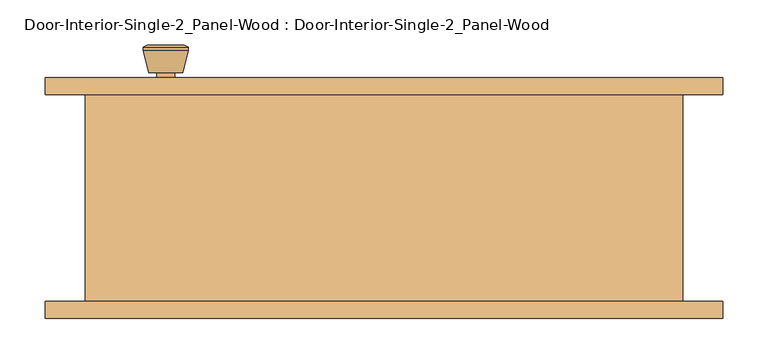
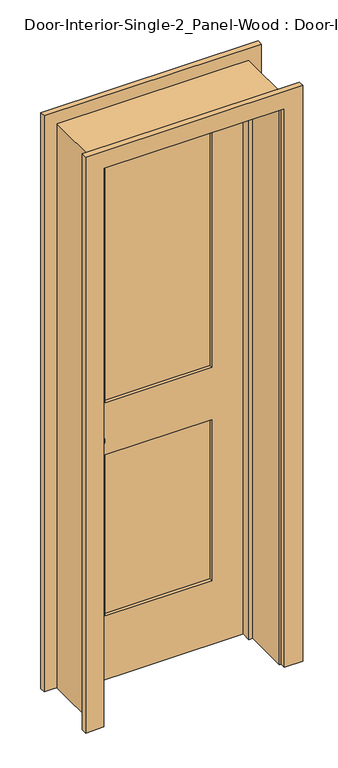
"""IFC4 building model written with IfcOpenShell, lengths in millimetres: door geometry, Door-Interior-Single-2_Panel-Wood : Door-Interior-Single-2_Panel-Wood."""

from ifc_helpers import new_model, si_unit, point, frame, frame_2d, origin, place, context, project, spatial, polyline, circle_curve, trimmed, segment, composite_curve, outline, extrude, faceted_brep, source, transform, mapped, element, save
from ifc_brep_helpers import plane_surface, cylinder_surface, revolved_surface, advanced_brep


def door_interior_single_2_panel_wood_door_interior_single_2_5f4e2ecc(model_context):
    return source(origin(), model_context, "Body", "SolidModel", [
        advanced_brep(
        [(-241.3, 70.2, 914.4), (-231.3, 70.2, 914.4), (-251.3, 70.2, 914.4), (-220.8241324, 21.2, 914.4), (-241.3, 21.2, 914.4), (-261.7758676, 21.2, 914.4), (-216.3, 23.0278681, 914.4), (-266.3, 23.0278681, 914.4), (-216.3, 26.4915463, 914.4), (-266.3, 26.4915463, 914.4), (-222.663764, 51.2, 914.4), (-259.936236, 51.2, 914.4), (-231.3, 51.2, 914.4), (-251.3, 51.2, 914.4)],
        [
            (0, 1),
            (1, 2, circle_curve(frame((-241.3, 70.2, 914.4), z_axis=(0.0, 1.0, 0.0), x_axis=(-1.0, 0.0, 0.0)), 10.0)),
            (2, 0),
            (2, 1, circle_curve(frame((-241.3, 70.2, 914.4), z_axis=(0.0, 1.0, 0.0), x_axis=(-1.0, 0.0, 0.0)), 10.0)),
            (3, 4),
            (4, 5),
            (5, 3, circle_curve(frame((-241.3, 21.2, 914.4), z_axis=(0.0, -1.0, 0.0), x_axis=(-1.0, 0.0, 0.0)), 20.4758676)),
            (3, 5, circle_curve(frame((-241.3, 21.2, 914.4), z_axis=(0.0, -1.0, 0.0), x_axis=(-1.0, 0.0, 0.0)), 20.4758676)),
            (6, 3),
            (5, 7),
            (7, 6, circle_curve(frame((-241.3, 23.0278681, 914.4), z_axis=(0.0, -1.0, 0.0), x_axis=(-1.0, 0.0, 0.0)), 25.0)),
            (6, 7, circle_curve(frame((-241.3, 23.0278681, 914.4), z_axis=(0.0, -1.0, 0.0), x_axis=(-1.0, 0.0, 0.0)), 25.0)),
            (8, 6),
            (7, 9),
            (9, 8, circle_curve(frame((-241.3, 26.4915463, 914.4), z_axis=(0.0, -1.0, 0.0), x_axis=(-1.0, 0.0, 0.0)), 25.0)),
            (8, 9, circle_curve(frame((-241.3, 26.4915463, 914.4), z_axis=(0.0, -1.0, 0.0), x_axis=(-1.0, 0.0, 0.0)), 25.0)),
            (10, 8),
            (9, 11),
            (11, 10, circle_curve(frame((-241.3, 51.2, 914.4), z_axis=(0.0, -1.0, 0.0), x_axis=(-1.0, 0.0, 0.0)), 18.636236)),
            (10, 11, circle_curve(frame((-241.3, 51.2, 914.4), z_axis=(0.0, -1.0, 0.0), x_axis=(-1.0, 0.0, 0.0)), 18.636236)),
            (12, 10),
            (11, 13),
            (13, 12, circle_curve(frame((-241.3, 51.2, 914.4), z_axis=(0.0, -1.0, 0.0), x_axis=(-1.0, 0.0, 0.0)), 10.0)),
            (12, 13, circle_curve(frame((-241.3, 51.2, 914.4), z_axis=(0.0, -1.0, 0.0), x_axis=(-1.0, 0.0, 0.0)), 10.0)),
            (1, 12),
            (13, 2),
        ],
        [
            plane_surface(frame((-241.3, 70.2, 914.4), z_axis=(0.0, 1.0, 0.0), x_axis=(-1.0, 0.0, 0.0))),
            plane_surface(frame((-241.3, 21.2, 914.4), z_axis=(0.0, -1.0, 0.0), x_axis=(-1.0, 0.0, 0.0))),
            revolved_surface(polyline([(-261.7758676, 21.2, 914.4), (-266.3, 23.0278681, 914.4)]), (-241.3, 70.2, 914.4), (0.0, 1.0, 0.0)),
            cylinder_surface(frame((-241.3, 70.2, 914.4), z_axis=(0.0, 1.0, 0.0), x_axis=(-1.0, 0.0, 0.0)), 25.0),
            revolved_surface(polyline([(-266.3, 26.4915463, 914.4), (-259.936236, 51.2, 914.4)]), (-241.3, 70.2, 914.4), (0.0, 1.0, 0.0)),
            plane_surface(frame((-241.3, 51.2, 914.4), z_axis=(0.0, 1.0, 0.0), x_axis=(-1.0, 0.0, 0.0))),
            cylinder_surface(frame((-241.3, 70.2, 914.4), z_axis=(0.0, 1.0, 0.0), x_axis=(-1.0, 0.0, 0.0)), 10.0),
        ],
        [
            (0, [[1, 2, 3]]),
            (0, [[-3, 4, -1]]),
            (1, [[5, 6, 7]]),
            (1, [[-6, -5, 8]]),
            (2, [[9, -7, 10, 11]]),
            (2, [[-10, -8, -9, 12]]),
            (3, [[13, -11, 14, 15]]),
            (3, [[-14, -12, -13, 16]]),
            (4, [[17, -15, 18, 19]]),
            (4, [[-18, -16, -17, 20]]),
            (5, [[21, -19, 22, 23]]),
            (5, [[-22, -20, -21, 24]]),
            (6, [[25, -23, 26, -2]]),
            (6, [[-26, -24, -25, -4]]),
        ],
    ),
        extrude(outline(composite_curve([segment(trimmed(circle_curve(frame_2d((914.4, -241.3)), 30.0), [point((914.4, -271.3))], [point((914.4, -211.3))], False, "CARTESIAN"), True, "CONTINUOUS"), segment(trimmed(circle_curve(frame_2d((914.4, -241.3)), 30.0), [point((914.4, -211.3))], [point((914.4, -271.3))], False, "CARTESIAN"), True, "CONTINUOUS")], self_intersect=False)), frame((0.0, 70.2, 0.0), z_axis=(0.0, 1.0, 0.0), x_axis=(0.0, 0.0, 1.0)), (0.0, 0.0, 1.0), 6.0),
        advanced_brep(
        [(-241.3, 117.125, 914.4), (-251.3, 117.125, 914.4), (-231.3, 117.125, 914.4), (-220.8241324, 166.125, 914.4), (-261.7758676, 166.125, 914.4), (-241.3, 166.125, 914.4), (-216.3, 164.2971319, 914.4), (-266.3, 164.2971319, 914.4), (-216.3, 160.8334537, 914.4), (-266.3, 160.8334537, 914.4), (-222.663764, 136.125, 914.4), (-259.936236, 136.125, 914.4), (-231.3, 136.125, 914.4), (-251.3, 136.125, 914.4)],
        [
            (0, 1),
            (1, 2, circle_curve(frame((-241.3, 117.125, 914.4), z_axis=(0.0, -1.0, 0.0), x_axis=(-1.0, 0.0, 0.0)), 10.0)),
            (2, 0),
            (2, 1, circle_curve(frame((-241.3, 117.125, 914.4), z_axis=(0.0, -1.0, 0.0), x_axis=(-1.0, 0.0, 0.0)), 10.0)),
            (3, 4, circle_curve(frame((-241.3, 166.125, 914.4), z_axis=(0.0, 1.0, 0.0), x_axis=(-1.0, 0.0, 0.0)), 20.4758676)),
            (4, 5),
            (5, 3),
            (4, 3, circle_curve(frame((-241.3, 166.125, 914.4), z_axis=(0.0, 1.0, 0.0), x_axis=(-1.0, 0.0, 0.0)), 20.4758676)),
            (6, 7, circle_curve(frame((-241.3, 164.2971319, 914.4), z_axis=(0.0, 1.0, 0.0), x_axis=(-1.0, 0.0, 0.0)), 25.0)),
            (7, 4),
            (3, 6),
            (7, 6, circle_curve(frame((-241.3, 164.2971319, 914.4), z_axis=(0.0, 1.0, 0.0), x_axis=(-1.0, 0.0, 0.0)), 25.0)),
            (8, 9, circle_curve(frame((-241.3, 160.8334537, 914.4), z_axis=(0.0, 1.0, 0.0), x_axis=(-1.0, 0.0, 0.0)), 25.0)),
            (9, 7),
            (6, 8),
            (9, 8, circle_curve(frame((-241.3, 160.8334537, 914.4), z_axis=(0.0, 1.0, 0.0), x_axis=(-1.0, 0.0, 0.0)), 25.0)),
            (10, 11, circle_curve(frame((-241.3, 136.125, 914.4), z_axis=(0.0, 1.0, 0.0), x_axis=(-1.0, 0.0, 0.0)), 18.636236)),
            (11, 9),
            (8, 10),
            (11, 10, circle_curve(frame((-241.3, 136.125, 914.4), z_axis=(0.0, 1.0, 0.0), x_axis=(-1.0, 0.0, 0.0)), 18.636236)),
            (12, 13, circle_curve(frame((-241.3, 136.125, 914.4), z_axis=(0.0, 1.0, 0.0), x_axis=(-1.0, 0.0, 0.0)), 10.0)),
            (13, 11),
            (10, 12),
            (13, 12, circle_curve(frame((-241.3, 136.125, 914.4), z_axis=(0.0, 1.0, 0.0), x_axis=(-1.0, 0.0, 0.0)), 10.0)),
            (1, 13),
            (12, 2),
        ],
        [
            plane_surface(frame((-241.3, 117.125, 914.4), z_axis=(0.0, -1.0, 0.0), x_axis=(-1.0, 0.0, 0.0))),
            plane_surface(frame((-241.3, 166.125, 914.4), z_axis=(0.0, 1.0, 0.0), x_axis=(-1.0, 0.0, 0.0))),
            revolved_surface(polyline([(-261.7758676, 166.125, 914.4), (-266.3, 164.2971319, 914.4)]), (-241.3, 117.125, 914.4), (0.0, -1.0, 0.0)),
            cylinder_surface(frame((-241.3, 117.125, 914.4), z_axis=(0.0, -1.0, 0.0), x_axis=(-1.0, 0.0, 0.0)), 25.0),
            revolved_surface(polyline([(-266.3, 160.8334537, 914.4), (-259.936236, 136.125, 914.4)]), (-241.3, 117.125, 914.4), (0.0, -1.0, 0.0)),
            plane_surface(frame((-241.3, 136.125, 914.4), z_axis=(0.0, -1.0, 0.0), x_axis=(-1.0, 0.0, 0.0))),
            cylinder_surface(frame((-241.3, 117.125, 914.4), z_axis=(0.0, -1.0, 0.0), x_axis=(-1.0, 0.0, 0.0)), 10.0),
        ],
        [
            (0, [[1, 2, 3]]),
            (0, [[-3, 4, -1]]),
            (1, [[5, 6, 7]]),
            (1, [[8, -7, -6]]),
            (2, [[9, 10, -5, 11]]),
            (2, [[12, -11, -8, -10]]),
            (3, [[13, 14, -9, 15]]),
            (3, [[16, -15, -12, -14]]),
            (4, [[17, 18, -13, 19]]),
            (4, [[20, -19, -16, -18]]),
            (5, [[21, 22, -17, 23]]),
            (5, [[24, -23, -20, -22]]),
            (6, [[-2, 25, -21, 26]]),
            (6, [[-4, -26, -24, -25]]),
        ],
    ),
        extrude(outline(composite_curve([segment(trimmed(circle_curve(frame_2d((914.4, -241.3)), 30.0), [point((914.4, -271.3))], [point((914.4, -211.3))], False, "CARTESIAN"), True, "CONTINUOUS"), segment(trimmed(circle_curve(frame_2d((914.4, -241.3)), 30.0), [point((914.4, -211.3))], [point((914.4, -271.3))], False, "CARTESIAN"), True, "CONTINUOUS")], self_intersect=False)), frame((0.0, 111.125, 0.0), z_axis=(0.0, 1.0, 0.0), x_axis=(0.0, 0.0, 1.0)), (0.0, 0.0, 1.0), 6.0),
        faceted_brep([(330.2, 111.125, 0.0), (330.2, -117.475, 0.0), (304.8, -117.475, 0.0), (304.8, 41.275, 0.0), (292.1, 41.275, 0.0), (292.1, 76.2, 0.0), (304.8, 76.2, 0.0), (304.8, 111.125, 0.0), (330.2, 111.125, 2057.4), (330.2, -117.475, 2057.4), (-330.2, -117.475, 2057.4), (-330.2, -117.475, 0.0), (-304.8, -117.475, 0.0), (-304.8, -117.475, 2032.0), (304.8, -117.475, 2032.0), (304.8, 41.275, 2032.0), (-304.8, 41.275, 2032.0), (-304.8, 41.275, 0.0), (-292.1, 41.275, 0.0), (-292.1, 41.275, 2019.3), (292.1, 41.275, 2019.3), (292.1, 76.2, 2019.3), (-292.1, 76.2, 2019.3), (-292.1, 76.2, 0.0), (-304.8, 76.2, 0.0), (-304.8, 76.2, 2032.0), (304.8, 76.2, 2032.0), (304.8, 111.125, 2032.0), (-304.8, 111.125, 2032.0), (-304.8, 111.125, 0.0), (-330.2, 111.125, 0.0), (-330.2, 111.125, 2057.4)], [[[0, 1, 2, 3, 4, 5, 6, 7]], [[1, 0, 8, 9]], [[2, 1, 9, 10, 11, 12, 13, 14]], [[3, 2, 14, 15]], [[4, 3, 15, 16, 17, 18, 19, 20]], [[5, 4, 20, 21]], [[6, 5, 21, 22, 23, 24, 25, 26]], [[7, 6, 26, 27]], [[0, 7, 27, 28, 29, 30, 31, 8]], [[9, 8, 31, 10]], [[15, 14, 13, 16]], [[21, 20, 19, 22]], [[27, 26, 25, 28]], [[30, 29, 24, 23, 18, 17, 12, 11]], [[10, 31, 30, 11]], [[16, 13, 12, 17]], [[22, 19, 18, 23]], [[28, 25, 24, 29]]]),
        extrude(outline(polyline([(2032.0, -304.8), (0.0, -304.8), (0.0, 304.8), (2032.0, 304.8), (2032.0, -304.8)]), holes=[polyline([(1912.9375, -184.15), (1912.9375, 184.15), (1009.65, 184.15), (1009.65, -184.15), (1912.9375, -184.15)]), polyline([(819.15, -184.15), (819.15, 184.15), (231.775, 184.15), (231.775, -184.15), (819.15, -184.15)])]), frame((0.0, 76.2, 0.0), z_axis=(0.0, 1.0, 0.0), x_axis=(0.0, 0.0, 1.0)), (0.0, 0.0, 1.0), 34.925),
        extrude(outline(polyline([(184.15, 87.8416667), (-184.15, 87.8416667), (-184.15, 99.4833333), (184.15, 99.4833333), (184.15, 87.8416667)])), frame((0.0, 0.0, 1009.65), z_axis=(0.0, 0.0, 1.0), x_axis=(1.0, 0.0, 0.0)), (0.0, 0.0, 1.0), 903.2875),
        extrude(outline(polyline([(184.15, 87.8416667), (-184.15, 87.8416667), (-184.15, 99.4833333), (184.15, 99.4833333), (184.15, 87.8416667)])), frame((0.0, 0.0, 231.775), z_axis=(0.0, 0.0, 1.0), x_axis=(1.0, 0.0, 0.0)), (0.0, 0.0, 1.0), 587.375),
        extrude(outline(polyline([(0.0, 311.15), (0.0, 374.65), (2101.85, 374.65), (2101.85, -374.65), (0.0, -374.65), (0.0, -311.15), (2038.35, -311.15), (2038.35, 311.15), (0.0, 311.15)])), frame((0.0, 111.125, 0.0), z_axis=(0.0, 1.0, 0.0), x_axis=(0.0, 0.0, 1.0)), (0.0, 0.0, 1.0), 19.05),
        extrude(outline(polyline([(0.0, 311.15), (0.0, 374.65), (2101.85, 374.65), (2101.85, -374.65), (0.0, -374.65), (0.0, -311.15), (2038.35, -311.15), (2038.35, 311.15), (0.0, 311.15)])), frame((0.0, -136.525, 0.0), z_axis=(0.0, 1.0, 0.0), x_axis=(0.0, 0.0, 1.0)), (0.0, 0.0, 1.0), 19.05),
    ])


if __name__ == "__main__":
    model = new_model("IFC4")
    model_context = context("Model", 3, world=origin())
    ifc_project = project(units=[si_unit("LENGTHUNIT", "METRE", prefix="MILLI")], contexts=[model_context])
    site = spatial("IfcSite", under=ifc_project)
    building = spatial("IfcBuilding", under=site)
    placement = place(None, origin())
    door_interior_single_2_panel_wood_door_interior_single_2_shape = door_interior_single_2_panel_wood_door_interior_single_2_5f4e2ecc(model_context)
    element("IfcDoor", 1, ObjectType="Door-Interior-Single-2_Panel-Wood : Door-Interior-Single-2_Panel-Wood", at=placement, inside=building, context=model_context, shape_type="MappedRepresentation", body=[
        mapped(door_interior_single_2_panel_wood_door_interior_single_2_shape, transform((0.0, 0.0, 0.0), x_axis=(1.0, 0.0, 0.0), y_axis=(0.0, 1.0, 0.0), z_axis=(0.0, 0.0, 1.0))),
    ])
    save(model, "model.ifc")

# Revit data of these elements
# Type "Door-Interior-Single-2_Panel-Wood : Door-Interior-Single-2_Panel-Wood"
#   Type Mark = "12"
#   Assembly Code = "C1020300"
#   Analytic Construction = "Wooden"
#   Top Rail = 0' - 4 11/16"
#   Thickness = 0' - 1 3/8"
#   Thermal Resistance (R) = 2.5876 (h·ft²·°F)/BTU
#   Swing Angle [instance default] = 90.00°
#   Stiles = 0' - 4 3/4"
#   Rough Width = 2' - 2"
#   Rough Height = 6' - 9"
#   Lock Rail = 0' - 7 1/2"
#   Height = 6' - 8"
#   Width = 2' - 0"
#   Heat Transfer Coefficient (U) = 0.3865 BTU/(h·ft²·°F)
#   Bottom Rail = 0' - 9 1/8"
#   Trim Material = Cherry
#   Panel Material = Cherry
#   Frame Material = Cherry
#   Door Handle Material = Aluminum
#   Visual Light Transmittance = 0
#   Solar Heat Gain Coefficient = 0
#   Wall Closure = (empty or 0)
#   Function = (empty or 0)
# Element 1 (IfcDoor, "Door-Interior-Single-2_Panel-Wood : Door-Interior-Single-2_Panel-Wood")
#   Materials on its faces: "Cherry", "Aluminum"
# Materials
#   "Cherry": class "Wood", colour RGB 226 177 128, transparency 0, Description = "Prunus Serotina", Cost = 0
#   "Aluminum": class "Metal", colour RGB 247 247 247, transparency 0, Description = "Aluminum 6061", Cost = 0
